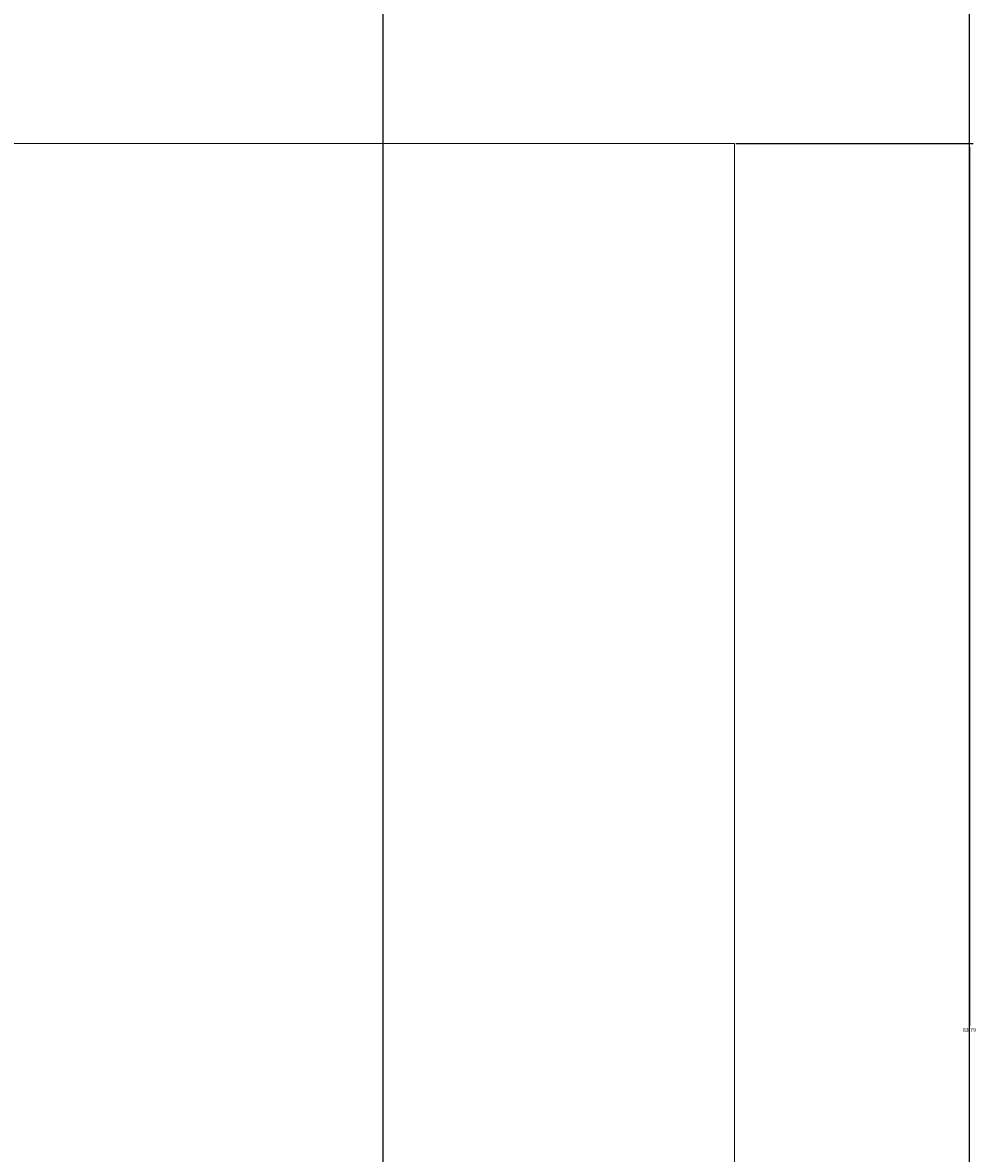
# Model space of a CAD drawing. Units: inches. Extents: x 412 to 584, y 208 to 437.
# Tile 14 of 28: x 539 to 584, y 262 to 315. Entities that reach past the tile are written whole.
import ezdxf

# ---------------------------------------------------------------- set-up
doc = ezdxf.new("R2010")
doc.units = ezdxf.units.IN
doc.header["$MEASUREMENT"] = 0
doc.layers.add('A-ANNO-DIMS', color=2, linetype='Continuous', lineweight=18)
doc.layers.add('E-ENCL', color=8, linetype='Continuous', lineweight=18)
doc.styles.get("Standard").update_dxf_attribs({"font": 'arial.ttf'})
doc.dimstyles.get("Standard").update_dxf_attribs({"dimtxt": 0.18, "dimasz": 0.18, "dimexe": 0.18, "dimexo": 0.0625, "dimgap": 0.09, "dimtad": 0, "dimtih": 1, "dimtoh": 1, "dimdec": 4, "dimzin": 0, "dimdsep": 46, "dimtxsty": 'Standard', "dimcen": 0.09, "dimadec": 0, "dimazin": 0, "dimtfac": 1, "dimtdec": 4, "dimtofl": 0, "dimtmove": 0, "dimatfit": 3, "dimfxl": 1, "dimtolj": 1, "dimtzin": 0, "dimarcsym": 0})

# ---------------------------------------------------------------- blocks, each defined once
blk = doc.blocks.new('*D17')
at = {"layer": 'A-ANNO-DIMS', "color": 0, "lineweight": -2, "transparency": 16777216}
for p, q in [((497.715, 426.185), (583.674, 426.185)), ((583.494, 426.005), (583.494, 323.031)), ((583.494, 219.693), (583.494, 322.667)), ((550.198, 219.513), (583.674, 219.513))]:
    blk.add_line(p, q, dxfattribs=at)
at = {"layer": 'A-ANNO-DIMS', "color": 0, "transparency": 16777216}
for points in [[(583.464, 426.005), (583.524, 426.005), (583.494, 426.185)], [(583.464, 219.693), (583.524, 219.693), (583.494, 219.513)]]:
    blk.add_solid(points, dxfattribs=at)
at = {"layer": 'Defpoints', "color": 0, "transparency": 16777216}
for p in [(497.652, 426.185), (550.135, 219.513), (583.494, 219.513)]:
    blk.add_point(p, dxfattribs=at)
at = {"layer": 'A-ANNO-DIMS', "color": 0, "transparency": 16777216, "insert": (583.494, 322.849), "char_height": 0.18, "attachment_point": 5}
blk.add_mtext('\\A1;206.67', dxfattribs=at)
blk = doc.blocks.new('*D18')
at = {"layer": 'A-ANNO-DIMS', "color": 0, "lineweight": -2, "transparency": 16777216}
for p, q in [((572.456, 309.377), (583.674, 309.377)), ((583.494, 309.197), (583.494, 267.665)), ((583.494, 225.768), (583.494, 267.301)), ((572.456, 225.588), (583.674, 225.588))]:
    blk.add_line(p, q, dxfattribs=at)
at = {"layer": 'A-ANNO-DIMS', "color": 0, "transparency": 16777216}
for points in [[(583.464, 309.197), (583.524, 309.197), (583.494, 309.377)], [(583.464, 225.768), (583.524, 225.768), (583.494, 225.588)]]:
    blk.add_solid(points, dxfattribs=at)
at = {"layer": 'Defpoints', "color": 0, "transparency": 16777216}
for p in [(572.394, 309.377), (572.394, 225.588), (583.494, 225.588)]:
    blk.add_point(p, dxfattribs=at)
at = {"layer": 'A-ANNO-DIMS', "color": 0, "transparency": 16777216, "insert": (583.494, 267.483), "char_height": 0.18, "attachment_point": 5}
blk.add_mtext('\\A1;83.79', dxfattribs=at)
blk = doc.blocks.new('*D28')
at = {"layer": 'A-ANNO-DIMS', "color": 0, "lineweight": -2, "transparency": 16777216}
for p, q in [((450.562, 256.635), (450.562, 437.465)), ((450.742, 437.285), (502.724, 437.285)), ((555.616, 437.285), (503.634, 437.285)), ((555.796, 256.635), (555.796, 437.465))]:
    blk.add_line(p, q, dxfattribs=at)
at = {"layer": 'A-ANNO-DIMS', "color": 0, "transparency": 16777216}
for points in [[(450.742, 437.315), (450.742, 437.255), (450.562, 437.285)], [(555.616, 437.315), (555.616, 437.255), (555.796, 437.285)]]:
    blk.add_solid(points, dxfattribs=at)
at = {"layer": 'Defpoints', "color": 0, "transparency": 16777216}
for p in [(555.796, 437.285), (450.562, 256.573), (555.796, 256.573)]:
    blk.add_point(p, dxfattribs=at)
at = {"layer": 'A-ANNO-DIMS', "color": 0, "transparency": 16777216, "insert": (503.179, 437.285), "char_height": 0.18, "attachment_point": 5}
blk.add_mtext('\\A1;105.23', dxfattribs=at)

msp = doc.modelspace()

# ---------------------------------------------------------------- linework, layer by layer
at = {"layer": 'E-ENCL'}
msp.add_lwpolyline([(423.5562, 309.3773), (572.3937, 309.3773), (572.3937, 225.5881), (423.5562, 225.5881)], close=True, dxfattribs=at)

# ---------------------------------------------------------------- dimensions: what is measured, and where the dimension line sits
at = {"layer": 'A-ANNO-DIMS'}
dim = msp.add_linear_dim(base=(555.7959, 437.2847), p1=(450.562, 256.5729), p2=(555.7959, 256.5729), dimstyle='Standard', override={"dimdec": 2, "dimlfac": 1, "dimrnd": 0, "dimzin": 0, "dimdsep": 46, "dimlunit": 2}, dxfattribs=at)
dim.commit()
dim.dimension.update_dxf_attribs({"geometry": '*D28', "text_midpoint": (503.1789, 437.2847)})
for base, p1, p2, picture, middle in [((583.4937, 219.5133), (497.6523, 426.1847), (550.1351, 219.5133), '*D17', (583.4937, 322.849)), ((583.4937, 225.5881), (572.3937, 309.3773), (572.3937, 225.5881), '*D18', (583.4937, 267.4827))]:
    dim = msp.add_linear_dim(base=base, p1=p1, p2=p2, angle=90, dimstyle='Standard', override={"dimdec": 2, "dimlfac": 1, "dimrnd": 0, "dimzin": 0, "dimdsep": 46, "dimlunit": 2}, dxfattribs=at)
    dim.commit()
    dim.dimension.update_dxf_attribs({"geometry": picture, "text_midpoint": middle})

doc.saveas('drawing.dxf')
